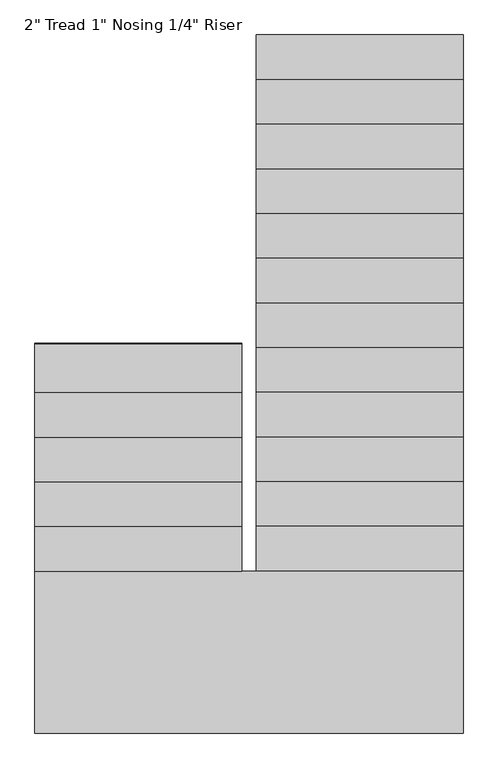
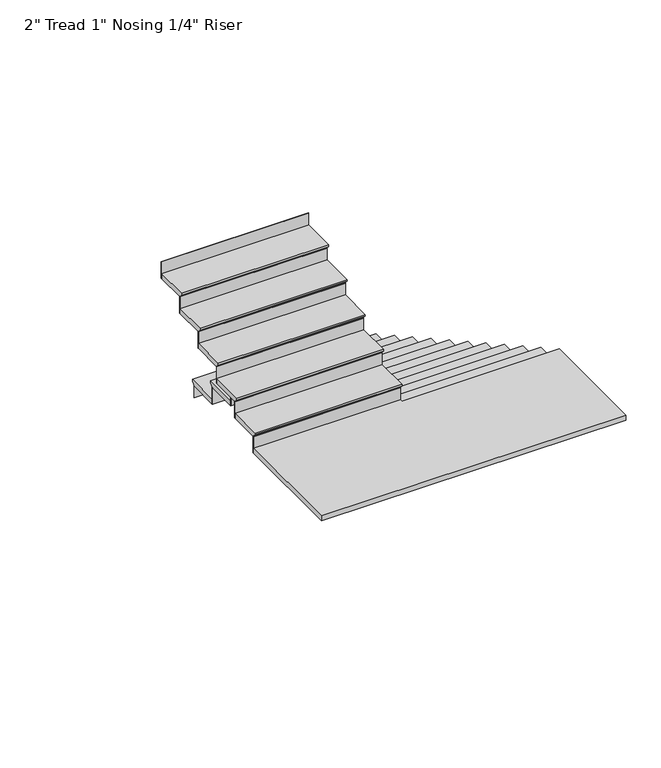
"""IFC4 building model written with IfcOpenShell, lengths in millimetres: stair flight geometry."""

from ifc_helpers import new_model, si_unit, origin, place, context, project, spatial, faceted_brep, source, transform, mapped, element, save


def stair_flight_7ee4923a(model_context):
    return source(origin(), model_context, "Body", "Brep", [
        faceted_brep([(-1578.560394, -1150.2831508, 150.2833333), (-1578.560394, -1150.2831508, 169.3333333), (-168.860394, -1150.2831508, 169.3333333), (-168.860394, -1150.2831508, 150.2833333), (-1578.560394, -1175.6831508, 124.8833333), (-168.860394, -1175.6831508, 124.8833333), (-1578.560394, -1480.4831508, 169.3333333), (-168.860394, -1480.4831508, 169.3333333), (-168.860394, -1175.6831508, 118.5333333), (-168.860394, -1480.4831508, 118.5333333), (-1578.560394, -1480.4831508, 118.5333333), (-1578.560394, -1175.6831508, 118.5333333)], [[[0, 1, 2, 3]], [[4, 0, 3, 5]], [[2, 1, 6, 7]], [[8, 9, 10, 11]], [[2, 7, 9, 8, 5, 3]], [[8, 11, 4, 5]], [[6, 1, 0, 4, 11, 10]], [[7, 6, 10, 9]]]),
        faceted_brep([(-1578.560394, -1175.6831508, 118.5333333), (-1578.560394, -1175.6831508, 0.0), (-1578.560394, -1182.0331508, 0.0), (-1578.560394, -1182.0331508, 118.5333333), (-168.860394, -1175.6831508, 118.5333333), (-168.860394, -1182.0331508, 118.5333333), (-168.860394, -1182.0331508, 0.0), (-168.860394, -1175.6831508, 0.0)], [[[0, 1, 2, 3]], [[4, 5, 6, 7]], [[1, 0, 4, 7]], [[2, 1, 7, 6]], [[3, 2, 6, 5]], [[0, 3, 5, 4]]]),
        faceted_brep([(-1578.560394, -1480.4831508, 287.8666667), (-1578.560394, -1480.4831508, 118.5333333), (-1578.560394, -1486.8331508, 118.5333333), (-1578.560394, -1486.8331508, 287.8666667), (-168.860394, -1480.4831508, 287.8666667), (-168.860394, -1486.8331508, 287.8666667), (-168.860394, -1486.8331508, 118.5333333), (-168.860394, -1480.4831508, 118.5333333)], [[[0, 1, 2, 3]], [[4, 5, 6, 7]], [[1, 0, 4, 7]], [[2, 1, 7, 6]], [[3, 2, 6, 5]], [[0, 3, 5, 4]]]),
        faceted_brep([(-168.860394, -1455.0831508, 338.6666667), (-1578.560394, -1455.0831508, 338.6666667), (-1578.560394, -1785.2831508, 338.6666667), (-168.860394, -1785.2831508, 338.6666667), (-168.860394, -1480.4831508, 287.8666667), (-168.860394, -1785.2831508, 287.8666667), (-1578.560394, -1785.2831508, 287.8666667), (-1578.560394, -1480.4831508, 287.8666667), (-168.860394, -1480.4831508, 294.2166667), (-168.860394, -1455.0831508, 319.6166667), (-1578.560394, -1480.4831508, 294.2166667), (-1578.560394, -1455.0831508, 319.6166667)], [[[0, 1, 2, 3]], [[4, 5, 6, 7]], [[0, 3, 5, 4, 8, 9]], [[4, 7, 10, 8]], [[2, 1, 11, 10, 7, 6]], [[3, 2, 6, 5]], [[11, 1, 0, 9]], [[10, 11, 9, 8]]]),
        faceted_brep([(-1578.560394, -1785.2831508, 457.2), (-1578.560394, -1785.2831508, 287.8666667), (-1578.560394, -1791.6331508, 287.8666667), (-1578.560394, -1791.6331508, 457.2), (-168.860394, -1785.2831508, 457.2), (-168.860394, -1791.6331508, 457.2), (-168.860394, -1791.6331508, 287.8666667), (-168.860394, -1785.2831508, 287.8666667)], [[[0, 1, 2, 3]], [[4, 5, 6, 7]], [[1, 0, 4, 7]], [[2, 1, 7, 6]], [[3, 2, 6, 5]], [[0, 3, 5, 4]]]),
        faceted_brep([(-168.860394, -1759.8831508, 508.0), (-1578.560394, -1759.8831508, 508.0), (-1578.560394, -2090.0831508, 508.0), (-168.860394, -2090.0831508, 508.0), (-168.860394, -1785.2831508, 457.2), (-168.860394, -2090.0831508, 457.2), (-1578.560394, -2090.0831508, 457.2), (-1578.560394, -1785.2831508, 457.2), (-168.860394, -1785.2831508, 463.55), (-168.860394, -1759.8831508, 488.95), (-1578.560394, -1785.2831508, 463.55), (-1578.560394, -1759.8831508, 488.95)], [[[0, 1, 2, 3]], [[4, 5, 6, 7]], [[0, 3, 5, 4, 8, 9]], [[4, 7, 10, 8]], [[2, 1, 11, 10, 7, 6]], [[3, 2, 6, 5]], [[11, 1, 0, 9]], [[10, 11, 9, 8]]]),
        faceted_brep([(-1578.560394, -2090.0831508, 626.5333333), (-1578.560394, -2090.0831508, 457.2), (-1578.560394, -2096.4331508, 457.2), (-1578.560394, -2096.4331508, 626.5333333), (-168.860394, -2090.0831508, 626.5333333), (-168.860394, -2096.4331508, 626.5333333), (-168.860394, -2096.4331508, 457.2), (-168.860394, -2090.0831508, 457.2)], [[[0, 1, 2, 3]], [[4, 5, 6, 7]], [[1, 0, 4, 7]], [[2, 1, 7, 6]], [[3, 2, 6, 5]], [[0, 3, 5, 4]]]),
        faceted_brep([(-168.860394, -2064.6831508, 677.3333333), (-1578.560394, -2064.6831508, 677.3333333), (-1578.560394, -2394.8831508, 677.3333333), (-168.860394, -2394.8831508, 677.3333333), (-168.860394, -2090.0831508, 626.5333333), (-168.860394, -2394.8831508, 626.5333333), (-1578.560394, -2394.8831508, 626.5333333), (-1578.560394, -2090.0831508, 626.5333333), (-168.860394, -2090.0831508, 632.8833333), (-168.860394, -2064.6831508, 658.2833333), (-1578.560394, -2090.0831508, 632.8833333), (-1578.560394, -2064.6831508, 658.2833333)], [[[0, 1, 2, 3]], [[4, 5, 6, 7]], [[0, 3, 5, 4, 8, 9]], [[4, 7, 10, 8]], [[2, 1, 11, 10, 7, 6]], [[3, 2, 6, 5]], [[11, 1, 0, 9]], [[10, 11, 9, 8]]]),
        faceted_brep([(-1578.560394, -2394.8831508, 795.8666667), (-1578.560394, -2394.8831508, 626.5333333), (-1578.560394, -2401.2331508, 626.5333333), (-1578.560394, -2401.2331508, 795.8666667), (-168.860394, -2394.8831508, 795.8666667), (-168.860394, -2401.2331508, 795.8666667), (-168.860394, -2401.2331508, 626.5333333), (-168.860394, -2394.8831508, 626.5333333)], [[[0, 1, 2, 3]], [[4, 5, 6, 7]], [[1, 0, 4, 7]], [[2, 1, 7, 6]], [[3, 2, 6, 5]], [[0, 3, 5, 4]]]),
        faceted_brep([(-168.860394, -2369.4831508, 846.6666667), (-1578.560394, -2369.4831508, 846.6666667), (-1578.560394, -2699.6831508, 846.6666667), (-168.860394, -2699.6831508, 846.6666667), (-168.860394, -2394.8831508, 795.8666667), (-168.860394, -2699.6831508, 795.8666667), (-1578.560394, -2699.6831508, 795.8666667), (-1578.560394, -2394.8831508, 795.8666667), (-168.860394, -2394.8831508, 802.2166667), (-168.860394, -2369.4831508, 827.6166667), (-1578.560394, -2394.8831508, 802.2166667), (-1578.560394, -2369.4831508, 827.6166667)], [[[0, 1, 2, 3]], [[4, 5, 6, 7]], [[0, 3, 5, 4, 8, 9]], [[4, 7, 10, 8]], [[2, 1, 11, 10, 7, 6]], [[3, 2, 6, 5]], [[11, 1, 0, 9]], [[10, 11, 9, 8]]]),
        faceted_brep([(-1578.560394, -2699.6831508, 965.2), (-1578.560394, -2699.6831508, 795.8666667), (-1578.560394, -2706.0331508, 795.8666667), (-1578.560394, -2706.0331508, 965.2), (-168.860394, -2699.6831508, 965.2), (-168.860394, -2706.0331508, 965.2), (-168.860394, -2706.0331508, 795.8666667), (-168.860394, -2699.6831508, 795.8666667)], [[[0, 1, 2, 3]], [[4, 5, 6, 7]], [[1, 0, 4, 7]], [[2, 1, 7, 6]], [[3, 2, 6, 5]], [[0, 3, 5, 4]]]),
        faceted_brep([(-168.860394, -2674.2831508, 1016.0), (-1578.560394, -2674.2831508, 1016.0), (-1578.560394, -3004.4831508, 1016.0), (-168.860394, -3004.4831508, 1016.0), (-168.860394, -2699.6831508, 965.2), (-168.860394, -3004.4831508, 965.2), (-1578.560394, -3004.4831508, 965.2), (-1578.560394, -2699.6831508, 965.2), (-168.860394, -2699.6831508, 971.55), (-168.860394, -2674.2831508, 996.95), (-1578.560394, -2699.6831508, 971.55), (-1578.560394, -2674.2831508, 996.95)], [[[0, 1, 2, 3]], [[4, 5, 6, 7]], [[0, 3, 5, 4, 8, 9]], [[4, 7, 10, 8]], [[2, 1, 11, 10, 7, 6]], [[3, 2, 6, 5]], [[11, 1, 0, 9]], [[10, 11, 9, 8]]]),
        faceted_brep([(-1578.560394, -3004.4831508, 1134.5333333), (-1578.560394, -3004.4831508, 965.2), (-1578.560394, -3010.8331508, 965.2), (-1578.560394, -3010.8331508, 1134.5333333), (-168.860394, -3004.4831508, 1134.5333333), (-168.860394, -3010.8331508, 1134.5333333), (-168.860394, -3010.8331508, 965.2), (-168.860394, -3004.4831508, 965.2)], [[[0, 1, 2, 3]], [[4, 5, 6, 7]], [[1, 0, 4, 7]], [[2, 1, 7, 6]], [[3, 2, 6, 5]], [[0, 3, 5, 4]]]),
        faceted_brep([(-168.860394, -2979.0831508, 1185.3333333), (-1578.560394, -2979.0831508, 1185.3333333), (-1578.560394, -3309.2831508, 1185.3333333), (-168.860394, -3309.2831508, 1185.3333333), (-168.860394, -3004.4831508, 1134.5333333), (-168.860394, -3309.2831508, 1134.5333333), (-1578.560394, -3309.2831508, 1134.5333333), (-1578.560394, -3004.4831508, 1134.5333333), (-168.860394, -3004.4831508, 1140.8833333), (-168.860394, -2979.0831508, 1166.2833333), (-1578.560394, -3004.4831508, 1140.8833333), (-1578.560394, -2979.0831508, 1166.2833333)], [[[0, 1, 2, 3]], [[4, 5, 6, 7]], [[0, 3, 5, 4, 8, 9]], [[4, 7, 10, 8]], [[2, 1, 11, 10, 7, 6]], [[3, 2, 6, 5]], [[11, 1, 0, 9]], [[10, 11, 9, 8]]]),
        faceted_brep([(-1578.560394, -3309.2831508, 1303.8666667), (-1578.560394, -3309.2831508, 1134.5333333), (-1578.560394, -3315.6331508, 1134.5333333), (-1578.560394, -3315.6331508, 1303.8666667), (-168.860394, -3309.2831508, 1303.8666667), (-168.860394, -3315.6331508, 1303.8666667), (-168.860394, -3315.6331508, 1134.5333333), (-168.860394, -3309.2831508, 1134.5333333)], [[[0, 1, 2, 3]], [[4, 5, 6, 7]], [[1, 0, 4, 7]], [[2, 1, 7, 6]], [[3, 2, 6, 5]], [[0, 3, 5, 4]]]),
        faceted_brep([(-168.860394, -3283.8831508, 1354.6666667), (-1578.560394, -3283.8831508, 1354.6666667), (-1578.560394, -3614.0831508, 1354.6666667), (-168.860394, -3614.0831508, 1354.6666667), (-168.860394, -3309.2831508, 1303.8666667), (-168.860394, -3614.0831508, 1303.8666667), (-1578.560394, -3614.0831508, 1303.8666667), (-1578.560394, -3309.2831508, 1303.8666667), (-168.860394, -3309.2831508, 1310.2166667), (-168.860394, -3283.8831508, 1335.6166667), (-1578.560394, -3309.2831508, 1310.2166667), (-1578.560394, -3283.8831508, 1335.6166667)], [[[0, 1, 2, 3]], [[4, 5, 6, 7]], [[0, 3, 5, 4, 8, 9]], [[4, 7, 10, 8]], [[2, 1, 11, 10, 7, 6]], [[3, 2, 6, 5]], [[11, 1, 0, 9]], [[10, 11, 9, 8]]]),
        faceted_brep([(-1578.560394, -3614.0831508, 1473.2), (-1578.560394, -3614.0831508, 1303.8666667), (-1578.560394, -3620.4331508, 1303.8666667), (-1578.560394, -3620.4331508, 1473.2), (-168.860394, -3614.0831508, 1473.2), (-168.860394, -3620.4331508, 1473.2), (-168.860394, -3620.4331508, 1303.8666667), (-168.860394, -3614.0831508, 1303.8666667)], [[[0, 1, 2, 3]], [[4, 5, 6, 7]], [[1, 0, 4, 7]], [[2, 1, 7, 6]], [[3, 2, 6, 5]], [[0, 3, 5, 4]]]),
        faceted_brep([(-168.860394, -3588.6831508, 1524.0), (-1578.560394, -3588.6831508, 1524.0), (-1578.560394, -3918.8831508, 1524.0), (-168.860394, -3918.8831508, 1524.0), (-168.860394, -3614.0831508, 1473.2), (-168.860394, -3918.8831508, 1473.2), (-1578.560394, -3918.8831508, 1473.2), (-1578.560394, -3614.0831508, 1473.2), (-168.860394, -3614.0831508, 1479.55), (-168.860394, -3588.6831508, 1504.95), (-1578.560394, -3614.0831508, 1479.55), (-1578.560394, -3588.6831508, 1504.95)], [[[0, 1, 2, 3]], [[4, 5, 6, 7]], [[0, 3, 5, 4, 8, 9]], [[4, 7, 10, 8]], [[2, 1, 11, 10, 7, 6]], [[3, 2, 6, 5]], [[11, 1, 0, 9]], [[10, 11, 9, 8]]]),
        faceted_brep([(-1578.560394, -3918.8831508, 1642.5333333), (-1578.560394, -3918.8831508, 1473.2), (-1578.560394, -3925.2331508, 1473.2), (-1578.560394, -3925.2331508, 1642.5333333), (-168.860394, -3918.8831508, 1642.5333333), (-168.860394, -3925.2331508, 1642.5333333), (-168.860394, -3925.2331508, 1473.2), (-168.860394, -3918.8831508, 1473.2)], [[[0, 1, 2, 3]], [[4, 5, 6, 7]], [[1, 0, 4, 7]], [[2, 1, 7, 6]], [[3, 2, 6, 5]], [[0, 3, 5, 4]]]),
        faceted_brep([(-168.860394, -3893.4831508, 1693.3333333), (-1578.560394, -3893.4831508, 1693.3333333), (-1578.560394, -4223.6831508, 1693.3333333), (-168.860394, -4223.6831508, 1693.3333333), (-168.860394, -3918.8831508, 1642.5333333), (-168.860394, -4223.6831508, 1642.5333333), (-1578.560394, -4223.6831508, 1642.5333333), (-1578.560394, -3918.8831508, 1642.5333333), (-168.860394, -3918.8831508, 1648.8833333), (-168.860394, -3893.4831508, 1674.2833333), (-1578.560394, -3918.8831508, 1648.8833333), (-1578.560394, -3893.4831508, 1674.2833333)], [[[0, 1, 2, 3]], [[4, 5, 6, 7]], [[0, 3, 5, 4, 8, 9]], [[4, 7, 10, 8]], [[2, 1, 11, 10, 7, 6]], [[3, 2, 6, 5]], [[11, 1, 0, 9]], [[10, 11, 9, 8]]]),
        faceted_brep([(-1578.560394, -4223.6831508, 1811.8666667), (-1578.560394, -4223.6831508, 1642.5333333), (-1578.560394, -4230.0331508, 1642.5333333), (-1578.560394, -4230.0331508, 1811.8666667), (-168.860394, -4223.6831508, 1811.8666667), (-168.860394, -4230.0331508, 1811.8666667), (-168.860394, -4230.0331508, 1642.5333333), (-168.860394, -4223.6831508, 1642.5333333)], [[[0, 1, 2, 3]], [[4, 5, 6, 7]], [[1, 0, 4, 7]], [[2, 1, 7, 6]], [[3, 2, 6, 5]], [[0, 3, 5, 4]]]),
        faceted_brep([(-168.860394, -4198.2831508, 1862.6666667), (-1578.560394, -4198.2831508, 1862.6666667), (-1578.560394, -4528.4831508, 1862.6666667), (-168.860394, -4528.4831508, 1862.6666667), (-168.860394, -4223.6831508, 1811.8666667), (-168.860394, -4528.4831508, 1811.8666667), (-1578.560394, -4528.4831508, 1811.8666667), (-1578.560394, -4223.6831508, 1811.8666667), (-168.860394, -4223.6831508, 1818.2166667), (-168.860394, -4198.2831508, 1843.6166667), (-1578.560394, -4223.6831508, 1818.2166667), (-1578.560394, -4198.2831508, 1843.6166667)], [[[0, 1, 2, 3]], [[4, 5, 6, 7]], [[0, 3, 5, 4, 8, 9]], [[4, 7, 10, 8]], [[2, 1, 11, 10, 7, 6]], [[3, 2, 6, 5]], [[11, 1, 0, 9]], [[10, 11, 9, 8]]]),
        faceted_brep([(-1578.560394, -4528.4831508, 1981.2), (-1578.560394, -4528.4831508, 1811.8666667), (-1578.560394, -4534.8331508, 1811.8666667), (-1578.560394, -4534.8331508, 1981.2), (-168.860394, -4528.4831508, 1981.2), (-168.860394, -4534.8331508, 1981.2), (-168.860394, -4534.8331508, 1811.8666667), (-168.860394, -4528.4831508, 1811.8666667)], [[[0, 1, 2, 3]], [[4, 5, 6, 7]], [[1, 0, 4, 7]], [[2, 1, 7, 6]], [[3, 2, 6, 5]], [[0, 3, 5, 4]]]),
        faceted_brep([(-168.860394, -4503.0831508, 2032.0), (-1578.560394, -4503.0831508, 2032.0), (-1578.560394, -4833.2831508, 2032.0), (-168.860394, -4833.2831508, 2032.0), (-168.860394, -4528.4831508, 1981.2), (-168.860394, -4833.2831508, 1981.2), (-1578.560394, -4833.2831508, 1981.2), (-1578.560394, -4528.4831508, 1981.2), (-168.860394, -4528.4831508, 1987.55), (-168.860394, -4503.0831508, 2012.95), (-1578.560394, -4528.4831508, 1987.55), (-1578.560394, -4503.0831508, 2012.95)], [[[0, 1, 2, 3]], [[4, 5, 6, 7]], [[0, 3, 5, 4, 8, 9]], [[4, 7, 10, 8]], [[2, 1, 11, 10, 7, 6]], [[3, 2, 6, 5]], [[11, 1, 0, 9]], [[10, 11, 9, 8]]]),
        faceted_brep([(-1578.560394, -4833.2831508, 2150.5333333), (-1578.560394, -4833.2831508, 1981.2), (-1578.560394, -4839.6331508, 1981.2), (-1578.560394, -4839.6331508, 2150.5333333), (-168.860394, -4833.2831508, 2150.5333333), (-168.860394, -4839.6331508, 2150.5333333), (-168.860394, -4839.6331508, 1981.2), (-168.860394, -4833.2831508, 1981.2)], [[[0, 1, 2, 3]], [[4, 5, 6, 7]], [[1, 0, 4, 7]], [[2, 1, 7, 6]], [[3, 2, 6, 5]], [[0, 3, 5, 4]]]),
        faceted_brep([(-3089.860394, -4782.4831508, 2201.3333333), (-3089.860394, -5912.7831508, 2201.3333333), (-168.860394, -5912.7831508, 2201.3333333), (-168.860394, -4807.8831508, 2201.3333333), (-1680.160394, -4807.8831508, 2201.3333333), (-1680.160394, -4782.4831508, 2201.3333333), (-3089.860394, -5912.7831508, 2150.5333333), (-3089.860394, -4782.4831508, 2150.5333333), (-1680.160394, -4782.4831508, 2150.5333333), (-1680.160394, -4807.8831508, 2150.5333333), (-1578.560394, -4807.8831508, 2150.5333333), (-1578.560394, -4833.2831508, 2150.5333333), (-168.860394, -4833.2831508, 2150.5333333), (-168.860394, -5912.7831508, 2150.5333333), (-168.860394, -4833.2831508, 2156.8833333), (-168.860394, -4807.8831508, 2182.2833333), (-1578.560394, -4833.2831508, 2156.8833333), (-1578.560394, -4807.8831508, 2182.2833333)], [[[0, 1, 2, 3, 4, 5]], [[6, 7, 8, 9, 10, 11, 12, 13]], [[1, 0, 7, 6]], [[2, 1, 6, 13]], [[3, 2, 13, 12, 14, 15]], [[12, 11, 16, 14]], [[11, 10, 17, 16]], [[4, 3, 15, 17, 10, 9]], [[5, 4, 9, 8]], [[0, 5, 8, 7]], [[15, 14, 16, 17]]]),
        faceted_brep([(-1680.160394, -4782.4831508, 2319.8666667), (-1680.160394, -4782.4831508, 2150.5333333), (-1680.160394, -4776.1331508, 2150.5333333), (-1680.160394, -4776.1331508, 2319.8666667), (-3089.860394, -4782.4831508, 2319.8666667), (-3089.860394, -4776.1331508, 2319.8666667), (-3089.860394, -4776.1331508, 2150.5333333), (-3089.860394, -4782.4831508, 2150.5333333)], [[[0, 1, 2, 3]], [[4, 5, 6, 7]], [[1, 0, 4, 7]], [[2, 1, 7, 6]], [[3, 2, 6, 5]], [[0, 3, 5, 4]]]),
        faceted_brep([(-3089.860394, -4807.8831508, 2370.6666667), (-1680.160394, -4807.8831508, 2370.6666667), (-1680.160394, -4477.6831508, 2370.6666667), (-3089.860394, -4477.6831508, 2370.6666667), (-3089.860394, -4782.4831508, 2319.8666667), (-3089.860394, -4477.6831508, 2319.8666667), (-1680.160394, -4477.6831508, 2319.8666667), (-1680.160394, -4782.4831508, 2319.8666667), (-3089.860394, -4782.4831508, 2326.2166667), (-3089.860394, -4807.8831508, 2351.6166667), (-1680.160394, -4782.4831508, 2326.2166667), (-1680.160394, -4807.8831508, 2351.6166667)], [[[0, 1, 2, 3]], [[4, 5, 6, 7]], [[0, 3, 5, 4, 8, 9]], [[4, 7, 10, 8]], [[2, 1, 11, 10, 7, 6]], [[3, 2, 6, 5]], [[11, 1, 0, 9]], [[10, 11, 9, 8]]]),
        faceted_brep([(-1680.160394, -4477.6831508, 2489.2), (-1680.160394, -4477.6831508, 2319.8666667), (-1680.160394, -4471.3331508, 2319.8666667), (-1680.160394, -4471.3331508, 2489.2), (-3089.860394, -4477.6831508, 2489.2), (-3089.860394, -4471.3331508, 2489.2), (-3089.860394, -4471.3331508, 2319.8666667), (-3089.860394, -4477.6831508, 2319.8666667)], [[[0, 1, 2, 3]], [[4, 5, 6, 7]], [[1, 0, 4, 7]], [[2, 1, 7, 6]], [[3, 2, 6, 5]], [[0, 3, 5, 4]]]),
        faceted_brep([(-3089.860394, -4503.0831508, 2540.0), (-1680.160394, -4503.0831508, 2540.0), (-1680.160394, -4172.8831508, 2540.0), (-3089.860394, -4172.8831508, 2540.0), (-3089.860394, -4477.6831508, 2489.2), (-3089.860394, -4172.8831508, 2489.2), (-1680.160394, -4172.8831508, 2489.2), (-1680.160394, -4477.6831508, 2489.2), (-3089.860394, -4477.6831508, 2495.55), (-3089.860394, -4503.0831508, 2520.95), (-1680.160394, -4477.6831508, 2495.55), (-1680.160394, -4503.0831508, 2520.95)], [[[0, 1, 2, 3]], [[4, 5, 6, 7]], [[0, 3, 5, 4, 8, 9]], [[4, 7, 10, 8]], [[2, 1, 11, 10, 7, 6]], [[3, 2, 6, 5]], [[11, 1, 0, 9]], [[10, 11, 9, 8]]]),
        faceted_brep([(-1680.160394, -4172.8831508, 2658.5333333), (-1680.160394, -4172.8831508, 2489.2), (-1680.160394, -4166.5331508, 2489.2), (-1680.160394, -4166.5331508, 2658.5333333), (-3089.860394, -4172.8831508, 2658.5333333), (-3089.860394, -4166.5331508, 2658.5333333), (-3089.860394, -4166.5331508, 2489.2), (-3089.860394, -4172.8831508, 2489.2)], [[[0, 1, 2, 3]], [[4, 5, 6, 7]], [[1, 0, 4, 7]], [[2, 1, 7, 6]], [[3, 2, 6, 5]], [[0, 3, 5, 4]]]),
        faceted_brep([(-3089.860394, -4198.2831508, 2709.3333333), (-1680.160394, -4198.2831508, 2709.3333333), (-1680.160394, -3868.0831508, 2709.3333333), (-3089.860394, -3868.0831508, 2709.3333333), (-3089.860394, -4172.8831508, 2658.5333333), (-3089.860394, -3868.0831508, 2658.5333333), (-1680.160394, -3868.0831508, 2658.5333333), (-1680.160394, -4172.8831508, 2658.5333333), (-3089.860394, -4172.8831508, 2664.8833333), (-3089.860394, -4198.2831508, 2690.2833333), (-1680.160394, -4172.8831508, 2664.8833333), (-1680.160394, -4198.2831508, 2690.2833333)], [[[0, 1, 2, 3]], [[4, 5, 6, 7]], [[0, 3, 5, 4, 8, 9]], [[4, 7, 10, 8]], [[2, 1, 11, 10, 7, 6]], [[3, 2, 6, 5]], [[11, 1, 0, 9]], [[10, 11, 9, 8]]]),
        faceted_brep([(-1680.160394, -3868.0831508, 2827.8666667), (-1680.160394, -3868.0831508, 2658.5333333), (-1680.160394, -3861.7331508, 2658.5333333), (-1680.160394, -3861.7331508, 2827.8666667), (-3089.860394, -3868.0831508, 2827.8666667), (-3089.860394, -3861.7331508, 2827.8666667), (-3089.860394, -3861.7331508, 2658.5333333), (-3089.860394, -3868.0831508, 2658.5333333)], [[[0, 1, 2, 3]], [[4, 5, 6, 7]], [[1, 0, 4, 7]], [[2, 1, 7, 6]], [[3, 2, 6, 5]], [[0, 3, 5, 4]]]),
        faceted_brep([(-3089.860394, -3893.4831508, 2878.6666667), (-1680.160394, -3893.4831508, 2878.6666667), (-1680.160394, -3563.2831508, 2878.6666667), (-3089.860394, -3563.2831508, 2878.6666667), (-3089.860394, -3868.0831508, 2827.8666667), (-3089.860394, -3563.2831508, 2827.8666667), (-1680.160394, -3563.2831508, 2827.8666667), (-1680.160394, -3868.0831508, 2827.8666667), (-3089.860394, -3868.0831508, 2834.2166667), (-3089.860394, -3893.4831508, 2859.6166667), (-1680.160394, -3868.0831508, 2834.2166667), (-1680.160394, -3893.4831508, 2859.6166667)], [[[0, 1, 2, 3]], [[4, 5, 6, 7]], [[0, 3, 5, 4, 8, 9]], [[4, 7, 10, 8]], [[2, 1, 11, 10, 7, 6]], [[3, 2, 6, 5]], [[11, 1, 0, 9]], [[10, 11, 9, 8]]]),
        faceted_brep([(-1680.160394, -3563.2831508, 2997.2), (-1680.160394, -3563.2831508, 2827.8666667), (-1680.160394, -3556.9331508, 2827.8666667), (-1680.160394, -3556.9331508, 2997.2), (-3089.860394, -3563.2831508, 2997.2), (-3089.860394, -3556.9331508, 2997.2), (-3089.860394, -3556.9331508, 2827.8666667), (-3089.860394, -3563.2831508, 2827.8666667)], [[[0, 1, 2, 3]], [[4, 5, 6, 7]], [[1, 0, 4, 7]], [[2, 1, 7, 6]], [[3, 2, 6, 5]], [[0, 3, 5, 4]]]),
        faceted_brep([(-1680.160394, -3258.4831508, 3166.5333333), (-1680.160394, -3258.4831508, 2997.2), (-1680.160394, -3252.1331508, 2997.2), (-1680.160394, -3252.1331508, 3166.5333333), (-3089.860394, -3258.4831508, 3166.5333333), (-3089.860394, -3252.1331508, 3166.5333333), (-3089.860394, -3252.1331508, 2997.2), (-3089.860394, -3258.4831508, 2997.2)], [[[0, 1, 2, 3]], [[4, 5, 6, 7]], [[1, 0, 4, 7]], [[2, 1, 7, 6]], [[3, 2, 6, 5]], [[0, 3, 5, 4]]]),
        faceted_brep([(-3089.860394, -3588.6831508, 3048.0), (-1680.160394, -3588.6831508, 3048.0), (-1680.160394, -3258.4831508, 3048.0), (-3089.860394, -3258.4831508, 3048.0), (-3089.860394, -3563.2831508, 2997.2), (-3089.860394, -3258.4831508, 2997.2), (-1680.160394, -3258.4831508, 2997.2), (-1680.160394, -3563.2831508, 2997.2), (-3089.860394, -3563.2831508, 3003.55), (-3089.860394, -3588.6831508, 3028.95), (-1680.160394, -3563.2831508, 3003.55), (-1680.160394, -3588.6831508, 3028.95)], [[[0, 1, 2, 3]], [[4, 5, 6, 7]], [[0, 3, 5, 4, 8, 9]], [[4, 7, 10, 8]], [[2, 1, 11, 10, 7, 6]], [[3, 2, 6, 5]], [[11, 1, 0, 9]], [[10, 11, 9, 8]]]),
    ])


if __name__ == "__main__":
    model = new_model("IFC4")
    model_context = context("Model", 3, world=origin())
    ifc_project = project(units=[si_unit("LENGTHUNIT", "METRE", prefix="MILLI")], contexts=[model_context])
    site = spatial("IfcSite", under=ifc_project)
    building = spatial("IfcBuilding", under=site)
    placement = place(None, origin())
    stair_flight_shape = stair_flight_7ee4923a(model_context)
    element("IfcStairFlight", 1, ObjectType="2\" Tread 1\" Nosing 1/4\" Riser", at=placement, inside=building, context=model_context, shape_type="MappedRepresentation", body=[
        mapped(stair_flight_shape, transform((0.0, 0.0, 0.0), x_axis=(1.0, 0.0, 0.0), y_axis=(0.0, 1.0, 0.0), z_axis=(0.0, 0.0, 1.0))),
    ])
    save(model, "model.ifc")
